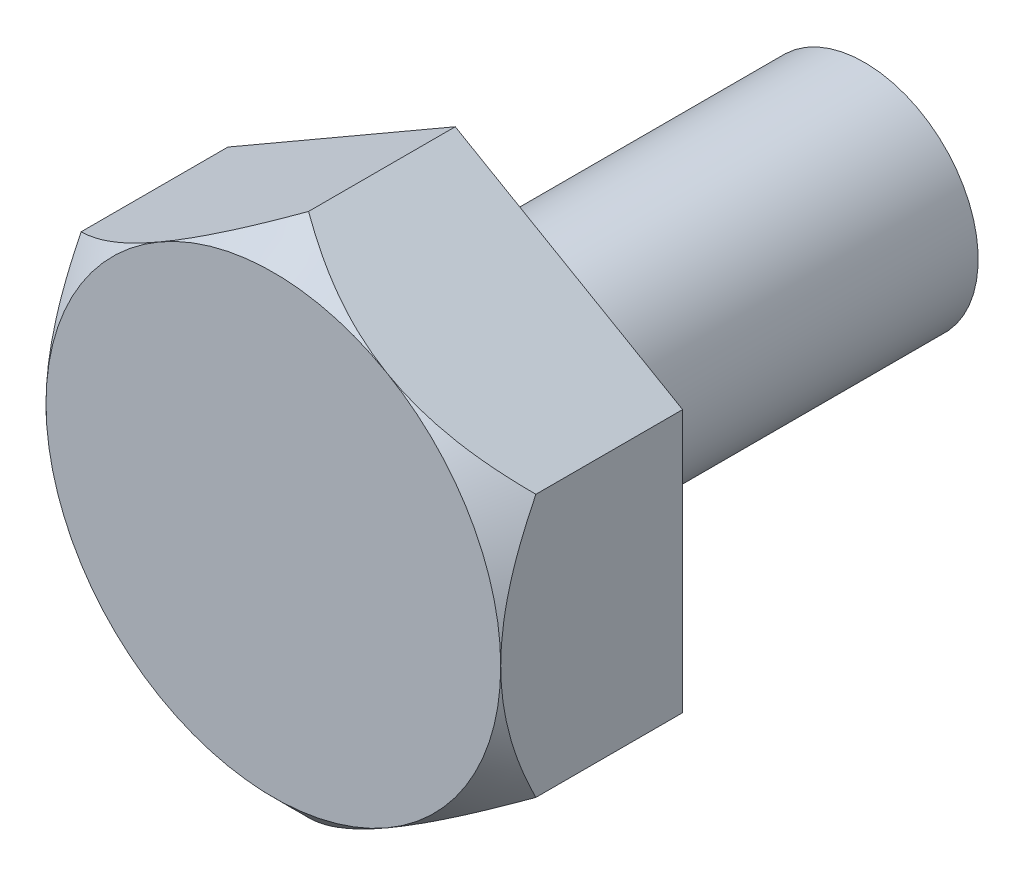
SolidWorks part; units mm, degrees
material "Plain Carbon Steel"
ref_plane "Front Plane" through (0, 0, 0) normal (0, 0, 1) x (1, 0, 0)
ref_plane "Top Plane" through (0, 0, 0) normal (0, 1, 0) x (1, 0, 0)
ref_plane "Right Plane" through (0, 0, 0) normal (1, 0, 0) x (0, 0, -1)
sketch "Hex Head Profile" plane through (0, 0, 0) normal (0, 0, 1) x (1, 0, 0)
  line L1 (5, -2.8868) -> (5, 2.8868)
  line L2 (5, 2.8868) -> (0, 5.7735)
  line L3 (0, 5.7735) -> (-5, 2.8868)
  line L4 (-5, 2.8868) -> (-5, -2.8868)
  line L5 (-5, -2.8868) -> (0, -5.7735)
  line L6 (0, -5.7735) -> (5, -2.8868)
  circle A0 centre (0, 0) radius 5 construction
  dimension "D1" = 10
extrude "Hex Head" add sketch "Hex Head Profile" along normal blind 4
sketch "Head Chamfer Profile" plane through (0, 0, 4) normal (0, 0, 1) x (1, 0, 0)
  line L0 (5, 2.8868) -> (0, 5.7735) construction
  circle A0 centre (0, 0) radius 5
extrude "Head Chamfer 45deg" cut sketch "Head Chamfer Profile" against normal blind 4 draft 45 flip side to cut
sketch "Shank Profile Ø5" plane through (0, 0, 0) normal (0, 0, -1) x (-1, 0, 0)
  circle A0 centre (0, 0) radius 2.5
  dimension "D1" = 5
extrude "Shank Ø5x9" add sketch "Shank Profile Ø5" along normal blind 9
